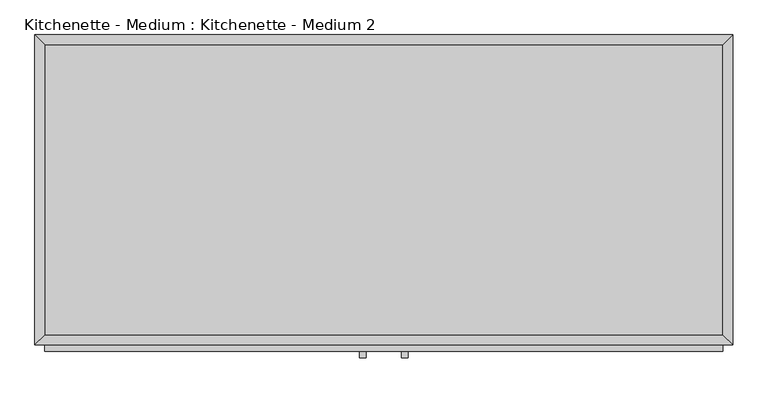
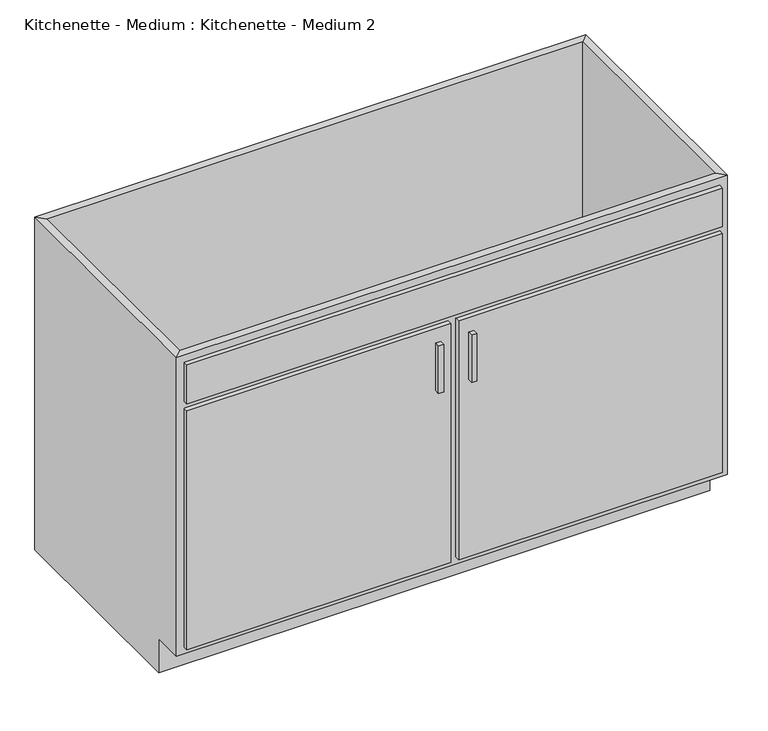
"""IFC4 building model written with IfcOpenShell, lengths in millimetres: proxy geometry, Kitchenette - Medium : Kitchenette - Medium 2."""

from ifc_helpers import new_model, si_unit, frame, origin, place, context, project, spatial, polyline, outline, extrude, faceted_brep, source, transform, mapped, element, save


def kitchenette_medium_kitchenette_medium_2_844211aa(model_context):
    return source(origin(), model_context, "Body", "SolidModel", [
        faceted_brep([(685.4877049, -590.55, 876.3), (685.4877049, -590.55, 88.9), (-648.0122951, -590.55, 88.9), (-648.0122951, -590.55, 876.3), (-667.0622951, -609.6, 876.3), (704.5377049, -609.6, 876.3), (-667.0622951, -609.6, 88.9), (704.5377049, -609.6, 88.9), (-648.0122951, -533.4, 88.9), (-648.0122951, -19.05, 88.9), (-648.0122951, -19.05, 876.3), (-667.0622951, 0.0, 876.3), (-667.0622951, 0.0, 0.0), (-667.0622951, -533.4, 0.0), (-667.0622951, -533.4, 88.9), (685.4877049, -19.05, 88.9), (685.4877049, -19.05, 876.3), (704.5377049, 0.0, 876.3), (704.5377049, 0.0, 0.0), (685.4877049, -533.4, 88.9), (704.5377049, -533.4, 88.9), (704.5377049, -533.4, 0.0)], [[[0, 1, 2, 3]], [[0, 3, 4, 5]], [[5, 4, 6, 7]], [[2, 1, 7, 6]], [[3, 2, 8, 9, 10]], [[4, 3, 10, 11]], [[6, 4, 11, 12, 13, 14]], [[2, 6, 14, 8]], [[10, 9, 15, 16]], [[11, 10, 16, 17]], [[12, 11, 17, 18]], [[1, 0, 16, 15, 19]], [[0, 5, 17, 16]], [[5, 7, 20, 21, 18, 17]], [[7, 1, 19, 20]], [[8, 19, 15, 9]], [[18, 21, 13, 12]], [[13, 21, 20, 19, 8, 14]]]),
        extrude(outline(polyline([(-16.1872951, -635.0), (-28.8872951, -635.0), (-28.8872951, -622.3), (-16.1872951, -622.3), (-16.1872951, -635.0)])), frame((0.0, 0.0, 573.769895), z_axis=(0.0, 0.0, 1.0), x_axis=(1.0, 0.0, 0.0)), (0.0, 0.0, 1.0), 124.730105),
        extrude(outline(polyline([(66.3627049, -635.0), (53.6627049, -635.0), (53.6627049, -622.3), (66.3627049, -622.3), (66.3627049, -635.0)])), frame((0.0, 0.0, 573.769895), z_axis=(0.0, 0.0, 1.0), x_axis=(1.0, 0.0, 0.0)), (0.0, 0.0, 1.0), 124.730105),
        extrude(outline(polyline([(685.4877049, -19.05), (685.4877049, -590.55), (-648.0122951, -590.55), (-648.0122951, -19.05), (685.4877049, -19.05)])), frame((0.0, 0.0, 88.9), z_axis=(0.0, 0.0, 1.0), x_axis=(1.0, 0.0, 0.0)), (0.0, 0.0, 1.0), 19.05),
        extrude(outline(polyline([(9.2127049, -622.3), (-648.0122951, -622.3), (-648.0122951, -609.6), (9.2127049, -609.6), (9.2127049, -622.3)])), frame((0.0, 0.0, 107.95), z_axis=(0.0, 0.0, 1.0), x_axis=(1.0, 0.0, 0.0)), (0.0, 0.0, 1.0), 628.65),
        extrude(outline(polyline([(685.4877049, -622.3), (28.2627049, -622.3), (28.2627049, -609.6), (685.4877049, -609.6), (685.4877049, -622.3)])), frame((0.0, 0.0, 107.95), z_axis=(0.0, 0.0, 1.0), x_axis=(1.0, 0.0, 0.0)), (0.0, 0.0, 1.0), 628.65),
        extrude(outline(polyline([(685.4877049, -622.3), (-648.0122951, -622.3), (-648.0122951, -609.6), (685.4877049, -609.6), (685.4877049, -622.3)])), frame((0.0, 0.0, 755.65), z_axis=(0.0, 0.0, 1.0), x_axis=(1.0, 0.0, 0.0)), (0.0, 0.0, 1.0), 101.6),
    ])


if __name__ == "__main__":
    model = new_model("IFC4")
    model_context = context("Model", 3, world=origin())
    ifc_project = project(units=[si_unit("LENGTHUNIT", "METRE", prefix="MILLI")], contexts=[model_context])
    site = spatial("IfcSite", under=ifc_project)
    building = spatial("IfcBuilding", under=site)
    placement = place(None, origin())
    kitchenette_medium_kitchenette_medium_2_shape = kitchenette_medium_kitchenette_medium_2_844211aa(model_context)
    element("IfcBuildingElementProxy", 1, Name="Kitchenette - Medium : Kitchenette - Medium 2", ObjectType="Kitchenette - Medium : Kitchenette - Medium 2", at=placement, inside=building, context=model_context, shape_type="MappedRepresentation", body=[
        mapped(kitchenette_medium_kitchenette_medium_2_shape, transform((0.0, 0.0, 0.0), x_axis=(1.0, 0.0, 0.0), y_axis=(0.0, 1.0, 0.0), z_axis=(0.0, 0.0, 1.0))),
    ])
    save(model, "model.ifc")

# Revit data of these elements
# Type "Kitchenette - Medium : Kitchenette - Medium 2"
#   Assembly Code = "E1090400"
#   Counter Length = 12' - 0"
#   Cabinet Width = 4' - 6"
#   Cabinet Height = 2' - 10 1/2"
#   Cabinet Depth = 2' - 0"
#   Toe Depth = 0' - 3"
#   Toe Height = 0' - 3 1/2"
#   Cabinet Material = Cabinets
#   Door/Drawer Material = Cabinets
#   Handle Material = Cabinets - Handles
#   Default Elevation = 0
# Element 1 (IfcBuildingElementProxy, "Kitchenette - Medium : Kitchenette - Medium 2")
#   Materials on its faces: "Cabinets", "Cabinets - Handles"
# Materials
#   "Cabinets": colour RGB 249 249 249, transparency 0
#   "Cabinets - Handles": class "Metal", colour RGB 57 57 57, transparency 0
